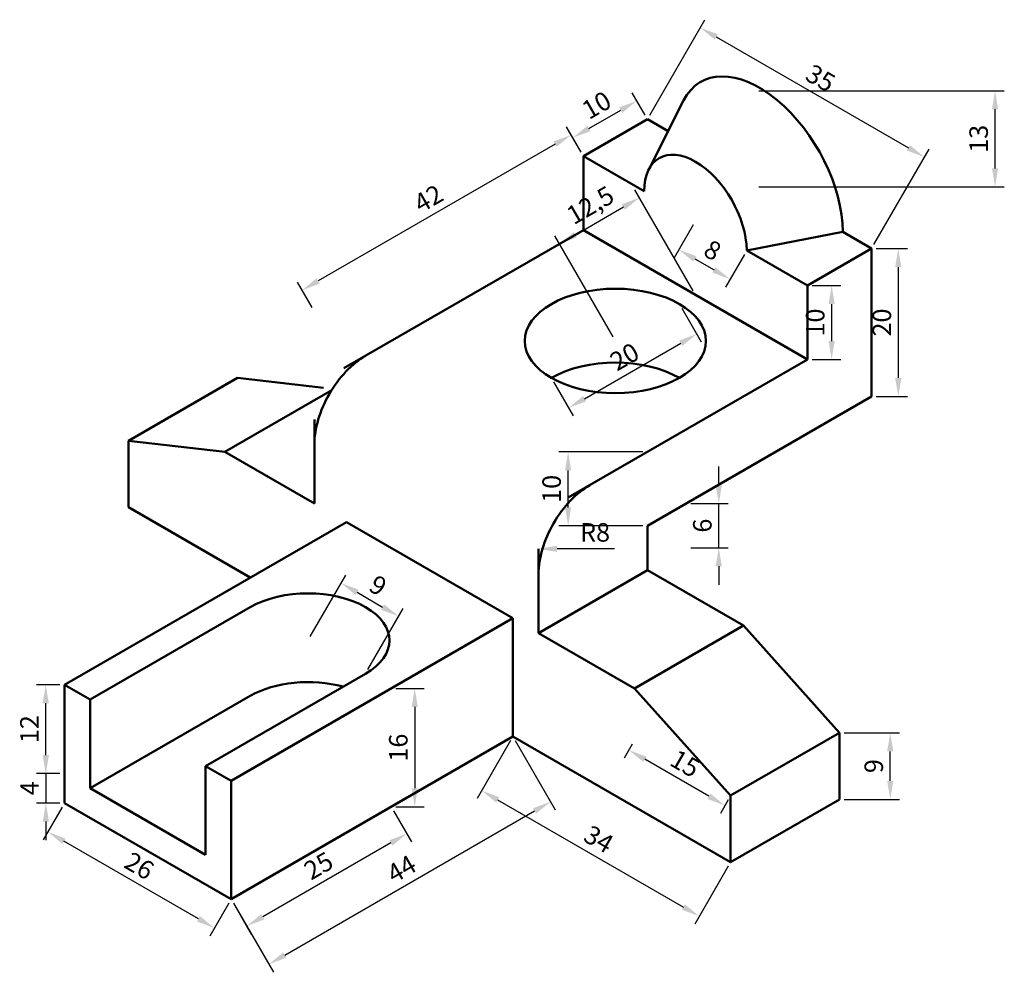
# Model space of a CAD drawing. Units: millimetres. Extents: x 1715 to 1848, y 1134 to 1263.
import ezdxf

# ---------------------------------------------------------------- set-up
doc = ezdxf.new("R2010")
doc.units = ezdxf.units.MM
doc.layers.add('M-DIMS', color=2, linetype='Continuous', lineweight=25)
doc.layers.add('M-OUTL', color=7, linetype='Continuous', lineweight=50)
doc.styles.get("Standard").update_dxf_attribs({"font": 'arial.ttf'})
doc.dimstyles.new('ISO-25', dxfattribs={"dimtxt": 2.5, "dimasz": 2.5, "dimexe": 1.25, "dimexo": 0.625, "dimtad": 1, "dimtxsty": 'Standard', "dimcen": 2.5, "dimadec": 0, "dimazin": 0, "dimtfac": 1, "dimtmove": 0, "dimatfit": 3, "dimfxl": 1, "dimarcsym": 0})

# ---------------------------------------------------------------- blocks, each defined once
blk = doc.blocks.new('*D1')
at = {"layer": 'Defpoints', "color": 0, "transparency": 16777216}
for p in [(1781.77, 1166.31), (1811.22, 1149.31), (1806.99, 1142)]:
    blk.add_point(p, dxfattribs=at)
at = {"layer": 'M-DIMS', "color": 0, "lineweight": -2, "transparency": 16777216}
for p, q in [((1781.46, 1165.77), (1776.92, 1157.92)), ((1779.71, 1157.75), (1804.83, 1143.25)), ((1810.9, 1148.77), (1806.37, 1140.92))]:
    blk.add_line(p, q, dxfattribs=at)
at = {"layer": 'M-DIMS', "color": 0, "transparency": 16777216}
for points in [[(1779.92, 1158.11), (1779.5, 1157.39), (1777.55, 1159)], [(1805.04, 1143.61), (1804.62, 1142.89), (1806.99, 1142)]]:
    blk.add_solid(points, dxfattribs=at)
at = {"layer": 'M-DIMS', "color": 0, "transparency": 16777216, "insert": (1793.22, 1152.15), "char_height": 2.5, "attachment_point": 5, "rotation": 330}
blk.add_mtext('34', dxfattribs=at)
blk = doc.blocks.new('*D2')
at = {"layer": 'Defpoints', "color": 0, "transparency": 16777216}
for p in [(1798.23, 1165.81), (1797.46, 1164.48), (1811.22, 1158.31)]:
    blk.add_point(p, dxfattribs=at)
at = {"layer": 'M-DIMS', "color": 0, "lineweight": -2, "transparency": 16777216}
for p, q in [((1797.91, 1165.27), (1796.83, 1163.4)), ((1808.28, 1158.23), (1799.62, 1163.23)), ((1810.9, 1157.77), (1809.82, 1155.9))]:
    blk.add_line(p, q, dxfattribs=at)
at = {"layer": 'M-DIMS', "color": 0, "transparency": 16777216}
for points in [[(1799.83, 1163.59), (1799.41, 1162.87), (1797.46, 1164.48)], [(1808.49, 1158.59), (1808.07, 1157.87), (1810.45, 1156.98)]]:
    blk.add_solid(points, dxfattribs=at)
at = {"layer": 'M-DIMS', "color": 0, "transparency": 16777216, "insert": (1804.9, 1162.38), "char_height": 2.5, "attachment_point": 5, "rotation": 330}
blk.add_mtext('15', dxfattribs=at)
blk = doc.blocks.new('*D3')
at = {"layer": 'Defpoints', "color": 0, "transparency": 16777216}
for p in [(1825.94, 1166.81), (1832.79, 1166.81), (1825.94, 1157.81)]:
    blk.add_point(p, dxfattribs=at)
at = {"layer": 'M-DIMS', "color": 0, "lineweight": -2, "transparency": 16777216}
for p, q in [((1826.56, 1166.81), (1834.04, 1166.81)), ((1832.79, 1160.31), (1832.79, 1164.31)), ((1826.56, 1157.81), (1834.04, 1157.81))]:
    blk.add_line(p, q, dxfattribs=at)
at = {"layer": 'M-DIMS', "color": 0, "transparency": 16777216}
for points in [[(1832.38, 1164.31), (1833.21, 1164.31), (1832.79, 1166.81)], [(1832.38, 1160.31), (1833.21, 1160.31), (1832.79, 1157.81)]]:
    blk.add_solid(points, dxfattribs=at)
at = {"layer": 'M-DIMS', "color": 0, "transparency": 16777216, "insert": (1830.89, 1162.31), "char_height": 2.5, "attachment_point": 5, "rotation": 90}
blk.add_mtext('9', dxfattribs=at)
blk = doc.blocks.new('*D4')
at = {"layer": 'Defpoints', "color": 0, "transparency": 16777216}
for p in [(1789.24, 1204.81), (1799.96, 1204.81), (1799.96, 1194.81)]:
    blk.add_point(p, dxfattribs=at)
at = {"layer": 'M-DIMS', "color": 0, "lineweight": -2, "transparency": 16777216}
for p, q in [((1799.33, 1204.81), (1787.99, 1204.81)), ((1789.24, 1197.31), (1789.24, 1202.31)), ((1799.33, 1194.81), (1787.99, 1194.81))]:
    blk.add_line(p, q, dxfattribs=at)
at = {"layer": 'M-DIMS', "color": 0, "transparency": 16777216}
for points in [[(1788.82, 1202.31), (1789.65, 1202.31), (1789.24, 1204.81)], [(1788.82, 1197.31), (1789.65, 1197.31), (1789.24, 1194.81)]]:
    blk.add_solid(points, dxfattribs=at)
at = {"layer": 'M-DIMS', "color": 0, "transparency": 16777216, "insert": (1787.33, 1199.81), "char_height": 2.5, "attachment_point": 5, "rotation": 90}
blk.add_mtext('10', dxfattribs=at)
blk = doc.blocks.new('*D5')
at = {"layer": 'Defpoints', "color": 0, "transparency": 16777216}
for p in [(1821.61, 1227.31), (1821.61, 1217.31), (1824.87, 1217.31)]:
    blk.add_point(p, dxfattribs=at)
at = {"layer": 'M-DIMS', "color": 0, "lineweight": -2, "transparency": 16777216}
for p, q in [((1822.23, 1227.31), (1826.12, 1227.31)), ((1824.87, 1224.81), (1824.87, 1219.81)), ((1822.23, 1217.31), (1826.12, 1217.31))]:
    blk.add_line(p, q, dxfattribs=at)
at = {"layer": 'M-DIMS', "color": 0, "transparency": 16777216}
for points in [[(1824.45, 1224.81), (1825.29, 1224.81), (1824.87, 1227.31)], [(1824.45, 1219.81), (1825.29, 1219.81), (1824.87, 1217.31)]]:
    blk.add_solid(points, dxfattribs=at)
at = {"layer": 'M-DIMS', "color": 0, "transparency": 16777216, "insert": (1822.97, 1222.31), "char_height": 2.5, "attachment_point": 5, "rotation": 90}
blk.add_mtext('10', dxfattribs=at)
blk = doc.blocks.new('*D6')
at = {"layer": 'Defpoints', "color": 0, "transparency": 16777216}
for p in [(1830.27, 1232.31), (1830.27, 1212.31), (1833.88, 1212.31)]:
    blk.add_point(p, dxfattribs=at)
at = {"layer": 'M-DIMS', "color": 0, "lineweight": -2, "transparency": 16777216}
for p, q in [((1830.89, 1232.31), (1835.13, 1232.31)), ((1833.88, 1229.81), (1833.88, 1214.81)), ((1830.89, 1212.31), (1835.13, 1212.31))]:
    blk.add_line(p, q, dxfattribs=at)
at = {"layer": 'M-DIMS', "color": 0, "transparency": 16777216}
for points in [[(1833.46, 1229.81), (1834.3, 1229.81), (1833.88, 1232.31)], [(1833.46, 1214.81), (1834.3, 1214.81), (1833.88, 1212.31)]]:
    blk.add_solid(points, dxfattribs=at)
at = {"layer": 'M-DIMS', "color": 0, "transparency": 16777216, "insert": (1831.98, 1222.31), "char_height": 2.5, "attachment_point": 5, "rotation": 90}
blk.add_mtext('20', dxfattribs=at)
blk = doc.blocks.new('*D7')
at = {"layer": 'Defpoints', "color": 0, "transparency": 16777216}
for p in [(1799.96, 1249.81), (1837.41, 1244.69), (1830.27, 1232.31)]:
    blk.add_point(p, dxfattribs=at)
at = {"layer": 'M-DIMS', "color": 0, "lineweight": -2, "transparency": 16777216}
for p, q in [((1800.27, 1250.36), (1807.73, 1263.27)), ((1809.27, 1260.94), (1835.25, 1245.94)), ((1830.58, 1232.86), (1838.04, 1245.77))]:
    blk.add_line(p, q, dxfattribs=at)
at = {"layer": 'M-DIMS', "color": 0, "transparency": 16777216}
for points in [[(1809.48, 1261.3), (1809.06, 1260.58), (1807.1, 1262.19)], [(1835.46, 1246.3), (1835.04, 1245.58), (1837.41, 1244.69)]]:
    blk.add_solid(points, dxfattribs=at)
at = {"layer": 'M-DIMS', "color": 0, "transparency": 16777216, "insert": (1823.21, 1255.09), "char_height": 2.5, "attachment_point": 5, "rotation": 330}
blk.add_mtext('35', dxfattribs=at)
blk = doc.blocks.new('*D8')
at = {"layer": 'Defpoints', "color": 0, "transparency": 16777216}
for p in [(1798.53, 1252.3), (1799.96, 1249.81), (1791.3, 1244.81)]:
    blk.add_point(p, dxfattribs=at)
at = {"layer": 'M-DIMS', "color": 0, "lineweight": -2, "transparency": 16777216}
for p, q in [((1799.65, 1250.36), (1797.9, 1253.38)), ((1792.03, 1248.55), (1796.36, 1251.05)), ((1790.99, 1245.36), (1789.24, 1248.38))]:
    blk.add_line(p, q, dxfattribs=at)
at = {"layer": 'M-DIMS', "color": 0, "transparency": 16777216}
for points in [[(1796.15, 1251.41), (1796.57, 1250.68), (1798.53, 1252.3)], [(1791.82, 1248.91), (1792.24, 1248.18), (1789.87, 1247.3)]]:
    blk.add_solid(points, dxfattribs=at)
at = {"layer": 'M-DIMS', "color": 0, "transparency": 16777216, "insert": (1793.24, 1251.44), "char_height": 2.5, "attachment_point": 5, "rotation": 30}
blk.add_mtext('10', dxfattribs=at)
blk = doc.blocks.new('*D9')
at = {"layer": 'Defpoints', "color": 0, "transparency": 16777216}
for p in [(1798.88, 1239.19), (1806.45, 1226.06), (1795.63, 1219.81)]:
    blk.add_point(p, dxfattribs=at)
at = {"layer": 'M-DIMS', "color": 0, "lineweight": -2, "transparency": 16777216}
for p, q in [((1806.14, 1226.61), (1798.25, 1240.27)), ((1790.22, 1234.19), (1796.71, 1237.94)), ((1795.32, 1220.36), (1787.43, 1234.02))]:
    blk.add_line(p, q, dxfattribs=at)
at = {"layer": 'M-DIMS', "color": 0, "transparency": 16777216}
for points in [[(1796.5, 1238.3), (1796.92, 1237.58), (1798.88, 1239.19)], [(1790.01, 1234.55), (1790.42, 1233.83), (1788.05, 1232.94)]]:
    blk.add_solid(points, dxfattribs=at)
at = {"layer": 'M-DIMS', "color": 0, "transparency": 16777216, "insert": (1792.4, 1237.91), "char_height": 2.5, "attachment_point": 5, "rotation": 30}
blk.add_mtext('12,5', dxfattribs=at)
blk = doc.blocks.new('*D10')
at = {"layer": 'Defpoints', "color": 0, "transparency": 16777216}
for p in [(1804.29, 1224.81), (1806.63, 1220.76), (1786.97, 1214.81)]:
    blk.add_point(p, dxfattribs=at)
at = {"layer": 'M-DIMS', "color": 0, "lineweight": -2, "transparency": 16777216}
for p, q in [((1804.6, 1224.27), (1807.25, 1219.68)), ((1791.47, 1212.01), (1804.46, 1219.51)), ((1787.28, 1214.27), (1789.93, 1209.68))]:
    blk.add_line(p, q, dxfattribs=at)
at = {"layer": 'M-DIMS', "color": 0, "transparency": 16777216}
for points in [[(1804.26, 1219.87), (1804.67, 1219.15), (1806.63, 1220.76)], [(1791.27, 1212.37), (1791.68, 1211.65), (1789.31, 1210.76)]]:
    blk.add_solid(points, dxfattribs=at)
at = {"layer": 'M-DIMS', "color": 0, "transparency": 16777216, "insert": (1797.02, 1217.41), "char_height": 2.5, "attachment_point": 5, "rotation": 30}
blk.add_mtext('20', dxfattribs=at)
blk = doc.blocks.new('*D11')
at = {"layer": 'Defpoints', "color": 0, "transparency": 16777216}
for p in [(1791.3, 1244.81), (1753.27, 1226.68), (1754.92, 1223.81)]:
    blk.add_point(p, dxfattribs=at)
at = {"layer": 'M-DIMS', "color": 0, "lineweight": -2, "transparency": 16777216}
for p, q in [((1790.99, 1245.36), (1789.02, 1248.77)), ((1787.48, 1246.43), (1755.43, 1227.93)), ((1754.61, 1224.36), (1752.64, 1227.77))]:
    blk.add_line(p, q, dxfattribs=at)
at = {"layer": 'M-DIMS', "color": 0, "transparency": 16777216}
for points in [[(1787.27, 1246.8), (1787.68, 1246.07), (1789.64, 1247.68)], [(1755.22, 1228.3), (1755.64, 1227.57), (1753.27, 1226.68)]]:
    blk.add_solid(points, dxfattribs=at)
at = {"layer": 'M-DIMS', "color": 0, "transparency": 16777216, "insert": (1770.51, 1238.81), "char_height": 2.5, "attachment_point": 5, "rotation": 30}
blk.add_mtext('42', dxfattribs=at)
blk = doc.blocks.new('*D12')
at = {"layer": 'Defpoints', "color": 0, "transparency": 16777216}
for p in [(1766.33, 1182.57), (1754.06, 1179.31), (1761.85, 1174.81)]:
    blk.add_point(p, dxfattribs=at)
at = {"layer": 'M-DIMS', "color": 0, "lineweight": -2, "transparency": 16777216}
for p, q in [((1754.37, 1179.86), (1759.16, 1188.15)), ((1760.7, 1185.82), (1764.16, 1183.82)), ((1762.17, 1175.36), (1766.95, 1183.65))]:
    blk.add_line(p, q, dxfattribs=at)
at = {"layer": 'M-DIMS', "color": 0, "transparency": 16777216}
for points in [[(1760.91, 1186.18), (1760.49, 1185.46), (1758.53, 1187.07)], [(1764.37, 1184.18), (1763.96, 1183.46), (1766.33, 1182.57)]]:
    blk.add_solid(points, dxfattribs=at)
at = {"layer": 'M-DIMS', "color": 0, "transparency": 16777216, "insert": (1763.38, 1186.46), "char_height": 2.5, "attachment_point": 5, "rotation": 330}
blk.add_mtext('9', dxfattribs=at)
blk = doc.blocks.new('*D13')
at = {"layer": 'Defpoints', "color": 0, "transparency": 16777216}
for p in [(1765.32, 1156.81), (1743.67, 1144.31), (1745.77, 1140.67)]:
    blk.add_point(p, dxfattribs=at)
at = {"layer": 'M-DIMS', "color": 0, "lineweight": -2, "transparency": 16777216}
for p, q in [((1765.63, 1156.27), (1768.05, 1152.08)), ((1765.26, 1151.92), (1747.94, 1141.92)), ((1743.98, 1143.77), (1746.4, 1139.58))]:
    blk.add_line(p, q, dxfattribs=at)
at = {"layer": 'M-DIMS', "color": 0, "transparency": 16777216}
for points in [[(1765.05, 1152.28), (1765.47, 1151.56), (1767.42, 1153.17)], [(1747.73, 1142.28), (1748.15, 1141.56), (1745.77, 1140.67)]]:
    blk.add_solid(points, dxfattribs=at)
at = {"layer": 'M-DIMS', "color": 0, "transparency": 16777216, "insert": (1755.65, 1148.56), "char_height": 2.5, "attachment_point": 5, "rotation": 30}
blk.add_mtext('25', dxfattribs=at)
blk = doc.blocks.new('*D14')
at = {"layer": 'Defpoints', "color": 0, "transparency": 16777216}
for p in [(1721.15, 1157.31), (1718.89, 1153.41), (1743.67, 1144.31)]:
    blk.add_point(p, dxfattribs=at)
at = {"layer": 'M-DIMS', "color": 0, "lineweight": -2, "transparency": 16777216}
for p, q in [((1720.84, 1156.77), (1718.27, 1152.32)), ((1739.24, 1141.66), (1721.06, 1152.16)), ((1743.35, 1143.77), (1740.78, 1139.32))]:
    blk.add_line(p, q, dxfattribs=at)
at = {"layer": 'M-DIMS', "color": 0, "transparency": 16777216}
for points in [[(1721.27, 1152.52), (1720.85, 1151.8), (1718.89, 1153.41)], [(1739.45, 1142.02), (1739.04, 1141.3), (1741.41, 1140.41)]]:
    blk.add_solid(points, dxfattribs=at)
at = {"layer": 'M-DIMS', "color": 0, "transparency": 16777216, "insert": (1731.1, 1148.55), "char_height": 2.5, "attachment_point": 5, "rotation": 330}
blk.add_mtext('26', dxfattribs=at)
blk = doc.blocks.new('*D15')
at = {"layer": 'Defpoints', "color": 0, "transparency": 16777216}
for p in [(1781.77, 1166.31), (1786.86, 1157.5), (1743.67, 1144.31)]:
    blk.add_point(p, dxfattribs=at)
at = {"layer": 'M-DIMS', "color": 0, "lineweight": -2, "transparency": 16777216}
for p, q in [((1782.08, 1165.77), (1787.48, 1156.42)), ((1750.92, 1136.75), (1784.69, 1156.25)), ((1743.98, 1143.77), (1749.38, 1134.42))]:
    blk.add_line(p, q, dxfattribs=at)
at = {"layer": 'M-DIMS', "color": 0, "transparency": 16777216}
for points in [[(1784.49, 1156.61), (1784.9, 1155.89), (1786.86, 1157.5)], [(1750.71, 1137.11), (1751.13, 1136.39), (1748.75, 1135.5)]]:
    blk.add_solid(points, dxfattribs=at)
at = {"layer": 'M-DIMS', "color": 0, "transparency": 16777216, "insert": (1766.87, 1148.13), "char_height": 2.5, "attachment_point": 5, "rotation": 30}
blk.add_mtext('44', dxfattribs=at)
blk = doc.blocks.new('*D16')
at = {"layer": 'Defpoints', "color": 0, "transparency": 16777216}
for p in [(1721.15, 1161.31), (1718.62, 1157.31), (1721.15, 1157.31)]:
    blk.add_point(p, dxfattribs=at)
at = {"layer": 'M-DIMS', "color": 0, "lineweight": -2, "transparency": 16777216}
for p, q in [((1718.62, 1163.81), (1718.62, 1166.31)), ((1720.52, 1161.31), (1717.37, 1161.31)), ((1718.62, 1161.31), (1718.62, 1157.31)), ((1720.52, 1157.31), (1717.37, 1157.31)), ((1718.62, 1154.81), (1718.62, 1152.31))]:
    blk.add_line(p, q, dxfattribs=at)
at = {"layer": 'M-DIMS', "color": 0, "transparency": 16777216}
for points in [[(1718.2, 1163.81), (1719.04, 1163.81), (1718.62, 1161.31)], [(1718.2, 1154.81), (1719.04, 1154.81), (1718.62, 1157.31)]]:
    blk.add_solid(points, dxfattribs=at)
at = {"layer": 'M-DIMS', "color": 0, "transparency": 16777216, "insert": (1716.74, 1159.31), "char_height": 2.5, "attachment_point": 5, "rotation": 90}
blk.add_mtext('4', dxfattribs=at)
blk = doc.blocks.new('*D17')
at = {"layer": 'Defpoints', "color": 0, "transparency": 16777216}
for p in [(1718.6, 1173.31), (1721.15, 1173.31), (1721.15, 1161.31)]:
    blk.add_point(p, dxfattribs=at)
at = {"layer": 'M-DIMS', "color": 0, "lineweight": -2, "transparency": 16777216}
for p, q in [((1720.52, 1173.31), (1717.35, 1173.31)), ((1718.6, 1163.81), (1718.6, 1170.81)), ((1720.52, 1161.31), (1717.35, 1161.31))]:
    blk.add_line(p, q, dxfattribs=at)
at = {"layer": 'M-DIMS', "color": 0, "transparency": 16777216}
for points in [[(1718.18, 1170.81), (1719.02, 1170.81), (1718.6, 1173.31)], [(1718.18, 1163.81), (1719.02, 1163.81), (1718.6, 1161.31)]]:
    blk.add_solid(points, dxfattribs=at)
at = {"layer": 'M-DIMS', "color": 0, "transparency": 16777216, "insert": (1716.72, 1167.31), "char_height": 2.5, "attachment_point": 5, "rotation": 90}
blk.add_mtext('12', dxfattribs=at)
blk = doc.blocks.new('*D18')
at = {"layer": 'Defpoints', "color": 0, "transparency": 16777216}
for p in [(1765.32, 1172.81), (1765.32, 1156.81), (1768.5, 1156.81)]:
    blk.add_point(p, dxfattribs=at)
at = {"layer": 'M-DIMS', "color": 0, "lineweight": -2, "transparency": 16777216}
for p, q in [((1765.94, 1172.81), (1769.75, 1172.81)), ((1768.5, 1170.31), (1768.5, 1159.31)), ((1765.94, 1156.81), (1769.75, 1156.81))]:
    blk.add_line(p, q, dxfattribs=at)
at = {"layer": 'M-DIMS', "color": 0, "transparency": 16777216}
for points in [[(1768.08, 1170.31), (1768.92, 1170.31), (1768.5, 1172.81)], [(1768.08, 1159.31), (1768.92, 1159.31), (1768.5, 1156.81)]]:
    blk.add_solid(points, dxfattribs=at)
at = {"layer": 'M-DIMS', "color": 0, "transparency": 16777216, "insert": (1766.6, 1164.81), "char_height": 2.5, "attachment_point": 5, "rotation": 90}
blk.add_mtext('16', dxfattribs=at)
blk = doc.blocks.new('*D19')
at = {"layer": 'Defpoints', "color": 0, "transparency": 16777216}
for p in [(1785.24, 1191.7), (1793.24, 1191.7)]:
    blk.add_point(p, dxfattribs=at)
at = {"layer": 'M-DIMS', "color": 0, "lineweight": -2, "transparency": 16777216}
blk.add_line((1795.52, 1191.7), (1787.74, 1191.7), dxfattribs=at)
at = {"layer": 'M-DIMS', "color": 0, "transparency": 16777216}
blk.add_solid([(1787.74, 1192.11), (1787.74, 1191.28), (1785.24, 1191.7)], dxfattribs=at)
at = {"layer": 'M-DIMS', "color": 0, "transparency": 16777216, "insert": (1792.88, 1193.6), "char_height": 2.5, "attachment_point": 5}
blk.add_mtext('R8', dxfattribs=at)
blk = doc.blocks.new('*D20')
at = {"layer": 'Defpoints', "color": 0, "transparency": 16777216}
for p in [(1806.45, 1236.06), (1813.38, 1232.06), (1811.13, 1228.17)]:
    blk.add_point(p, dxfattribs=at)
at = {"layer": 'M-DIMS', "color": 0, "lineweight": -2, "transparency": 16777216}
for p, q in [((1806.14, 1235.52), (1803.58, 1231.08)), ((1813.07, 1231.52), (1810.51, 1227.08)), ((1806.37, 1230.92), (1808.97, 1229.42))]:
    blk.add_line(p, q, dxfattribs=at)
at = {"layer": 'M-DIMS', "color": 0, "transparency": 16777216}
for points in [[(1806.58, 1231.28), (1806.16, 1230.56), (1804.2, 1232.17)], [(1809.17, 1229.78), (1808.76, 1229.06), (1811.13, 1228.17)]]:
    blk.add_solid(points, dxfattribs=at)
at = {"layer": 'M-DIMS', "color": 0, "transparency": 16777216, "insert": (1808.62, 1231.81), "char_height": 2.5, "attachment_point": 5, "rotation": 330}
blk.add_mtext('8', dxfattribs=at)
blk = doc.blocks.new('*D21')
at = {"layer": 'Defpoints', "color": 0, "transparency": 16777216}
for p in [(1814.41, 1253.66), (1846.97, 1253.66), (1814.41, 1240.66)]:
    blk.add_point(p, dxfattribs=at)
at = {"layer": 'M-DIMS', "color": 0, "lineweight": -2, "transparency": 16777216}
for p, q in [((1815.04, 1253.66), (1848.22, 1253.66)), ((1846.97, 1243.16), (1846.97, 1251.16)), ((1815.04, 1240.66), (1848.22, 1240.66))]:
    blk.add_line(p, q, dxfattribs=at)
at = {"layer": 'M-DIMS', "color": 0, "transparency": 16777216}
for points in [[(1846.55, 1251.16), (1847.38, 1251.16), (1846.97, 1253.66)], [(1846.55, 1243.16), (1847.38, 1243.16), (1846.97, 1240.66)]]:
    blk.add_solid(points, dxfattribs=at)
at = {"layer": 'M-DIMS', "color": 0, "transparency": 16777216, "insert": (1845.07, 1247.16), "char_height": 2.5, "attachment_point": 5, "rotation": 90}
blk.add_mtext('13', dxfattribs=at)
blk = doc.blocks.new('*D22')
at = {"layer": 'Defpoints', "color": 0, "transparency": 16777216}
for p in [(1805.2, 1197.84), (1809.61, 1197.84), (1805.2, 1191.84)]:
    blk.add_point(p, dxfattribs=at)
at = {"layer": 'M-DIMS', "color": 0, "lineweight": -2, "transparency": 16777216}
for p, q in [((1809.61, 1200.34), (1809.61, 1202.84)), ((1805.82, 1197.84), (1810.86, 1197.84)), ((1809.61, 1191.84), (1809.61, 1197.84)), ((1805.82, 1191.84), (1810.86, 1191.84)), ((1809.61, 1189.34), (1809.61, 1186.84))]:
    blk.add_line(p, q, dxfattribs=at)
at = {"layer": 'M-DIMS', "color": 0, "transparency": 16777216}
for points in [[(1809.19, 1200.34), (1810.03, 1200.34), (1809.61, 1197.84)], [(1809.19, 1189.34), (1810.03, 1189.34), (1809.61, 1191.84)]]:
    blk.add_solid(points, dxfattribs=at)
at = {"layer": 'M-DIMS', "color": 0, "transparency": 16777216, "insert": (1807.71, 1194.84), "char_height": 2.5, "attachment_point": 5, "rotation": 90}
blk.add_mtext('6', dxfattribs=at)

msp = doc.modelspace()

# ---------------------------------------------------------------- linework, layer by layer
at = {"layer": 'M-OUTL'}
for p, q in [((1800.139, 1243.002), (1804.852, 1252.338)), ((1799.958, 1249.815), (1791.298, 1244.815)), ((1802.761, 1248.196), (1799.958, 1249.815)), ((1791.298, 1234.815), (1791.298, 1244.815)), ((1799.525, 1240.065), (1791.298, 1244.815)), ((1791.298, 1234.815), (1758.925, 1216.124)), ((1821.609, 1217.315), (1791.298, 1234.815)), ((1813.381, 1232.065), (1826.372, 1234.565)), ((1830.269, 1232.315), (1826.372, 1234.565)), ((1821.609, 1227.315), (1813.381, 1232.065)), ((1821.609, 1227.315), (1830.269, 1232.315)), ((1830.269, 1232.315), (1830.269, 1212.315)), ((1821.609, 1217.315), (1821.609, 1227.315)), ((1789.236, 1198.624), (1821.609, 1217.315)), ((1744.532, 1214.815), (1729.81, 1206.315)), ((1756.163, 1213.472), (1744.532, 1214.815)), ((1742.8, 1204.815), (1757.27, 1213.169)), ((1742.8, 1204.815), (1755.486, 1212.138)), ((1830.269, 1212.315), (1799.958, 1194.815)), ((1754.925, 1209.196), (1754.925, 1197.815)), ((1729.81, 1197.315), (1729.81, 1206.315)), ((1729.81, 1206.315), (1742.8, 1204.815)), ((1754.925, 1197.815), (1742.8, 1204.815)), ((1746.264, 1187.815), (1729.81, 1197.315)), ((1721.15, 1173.315), (1759.255, 1195.315)), ((1781.771, 1182.315), (1759.255, 1195.315)), ((1799.958, 1194.815), (1799.958, 1188.815)), ((1785.236, 1180.315), (1785.236, 1191.696)), ((1785.236, 1180.315), (1799.958, 1188.815)), ((1812.948, 1181.315), (1799.958, 1188.815)), ((1743.666, 1160.315), (1781.771, 1182.315)), ((1781.771, 1182.315), (1781.771, 1166.315)), ((1781.771, 1182.315), (1781.771, 1182.315)), ((1798.226, 1172.815), (1812.948, 1181.315)), ((1825.939, 1166.815), (1812.948, 1181.315)), ((1785.236, 1180.315), (1798.226, 1172.815)), ((1740.202, 1162.315), (1761.853, 1174.815)), ((1721.15, 1161.315), (1721.15, 1173.315)), ((1721.15, 1173.315), (1724.614, 1171.315)), ((1724.614, 1159.315), (1746.264, 1171.815)), ((1798.226, 1172.815), (1811.216, 1158.315)), ((1724.614, 1171.315), (1724.614, 1159.315)), ((1743.666, 1144.315), (1781.771, 1166.315)), ((1781.771, 1166.315), (1811.216, 1149.315)), ((1811.216, 1158.315), (1825.939, 1166.815)), ((1825.939, 1166.815), (1825.939, 1157.815)), ((1740.202, 1150.315), (1740.202, 1162.315)), ((1740.202, 1162.315), (1743.666, 1160.315)), ((1721.15, 1157.315), (1721.15, 1161.315)), ((1743.666, 1160.315), (1743.666, 1144.315)), ((1724.614, 1159.315), (1740.202, 1150.315)), ((1811.216, 1149.315), (1811.216, 1158.315)), ((1743.666, 1144.315), (1721.15, 1157.315)), ((1825.939, 1157.815), (1811.216, 1149.315))]:
    msp.add_line(p, q, dxfattribs=at)
msp.add_lwpolyline([(1724.614, 1171.315), (1746.264, 1183.815)], dxfattribs=at)
for centre, major_axis, start_param, end_param in [((1815.113, 1241.065), (7.961, -13.789), 0.7853982, 3.5029598), ((1806.453, 1236.065), (4.899, -8.485), 0.7853982, 3.9269908), ((1761.852, 1209.815), (-4.899, -8.485), 3.9269286, 5.4978493), ((1795.628, 1209.815), (12.247, 0), 0.7853982, 2.3561945), ((1792.163, 1192.315), (-4.899, -8.485), 3.9269286, 5.4978493), ((1754.059, 1179.315), (-11.023, 0), 2.3561945, 5.4977871), ((1754.059, 1167.315), (-11.023, 0), 4.2668277, 5.4977871)]:
    msp.add_ellipse(centre, major_axis=major_axis, ratio=0.5773503, start_param=start_param, end_param=end_param, dxfattribs=at)
msp.add_ellipse((1795.628, 1219.815), major_axis=(-12.247, 0), ratio=0.5773503, dxfattribs=at)

# ---------------------------------------------------------------- dimensions: what is measured, and where the dimension line sits
at = {"layer": 'M-DIMS'}
for p1, p2, distance, picture, middle in [((1799.958, 1249.815), (1830.269, 1232.315), 14.289, '*D7', (1823.209, 1255.086)), ((1791.298, 1244.815), (1799.958, 1249.815), 2.864, '*D8', (1793.245, 1251.442)), ((1791.298, 1244.815), (1754.925, 1223.815), -3.314, '*D11', (1770.514, 1238.813)), ((1795.628, 1219.815), (1806.453, 1226.065), 15.155, '*D9', (1792.399, 1237.907)), ((1806.453, 1236.065), (1813.381, 1232.065), -4.5, '*D20', (1808.618, 1231.814)), ((1786.968, 1214.815), (1804.288, 1224.815), -4.683, '*D10', (1797.018, 1217.406)), ((1754.059, 1179.315), (1761.853, 1174.815), 8.952, '*D12', (1763.383, 1186.464)), ((1743.666, 1144.315), (1781.771, 1166.315), -10.174, '*D15', (1766.869, 1148.127)), ((1781.771, 1166.315), (1811.216, 1149.315), -8.447, '*D1', (1793.222, 1152.147)), ((1811.216, 1158.315), (1798.226, 1165.815), 1.54, '*D2', (1804.902, 1162.377)), ((1743.666, 1144.315), (1721.15, 1157.315), 4.513, '*D14', (1731.102, 1148.553)), ((1765.317, 1156.815), (1743.666, 1144.315), 4.213, '*D13', (1755.647, 1148.563))]:
    dim = msp.add_aligned_dim(p1=p1, p2=p2, distance=distance, dimstyle='ISO-25', override={"dimclrd": 0, "dimclre": 0, "dimclrt": 0}, dxfattribs=at)
    dim.commit()
    dim.dimension.update_dxf_attribs({"geometry": picture, "text_midpoint": middle})
for base, p1, p2, picture, middle in [((1846.968, 1253.661), (1814.414, 1240.661), (1814.414, 1253.661), '*D21', (1845.065, 1247.161)), ((1833.882, 1212.315), (1830.269, 1232.315), (1830.269, 1212.315), '*D6', (1831.98, 1222.315)), ((1824.87, 1217.315), (1821.609, 1227.315), (1821.609, 1217.315), '*D5', (1822.969, 1222.315)), ((1789.236, 1204.815), (1799.958, 1194.815), (1799.958, 1204.815), '*D4', (1787.334, 1199.815)), ((1809.609, 1197.84), (1805.198, 1191.84), (1805.198, 1197.84), '*D22', (1807.707, 1194.84)), ((1718.601, 1173.315), (1721.15, 1161.315), (1721.15, 1173.315), '*D17', (1716.721, 1167.315)), ((1768.501, 1156.815), (1765.317, 1172.815), (1765.317, 1156.815), '*D18', (1766.6, 1164.815)), ((1718.618, 1157.315), (1721.15, 1161.315), (1721.15, 1157.315), '*D16', (1716.743, 1159.315)), ((1832.793, 1166.815), (1825.939, 1157.815), (1825.939, 1166.815), '*D3', (1830.891, 1162.315))]:
    dim = msp.add_linear_dim(base=base, p1=p1, p2=p2, angle=90, dimstyle='ISO-25', override={"dimclrd": 0, "dimclre": 0, "dimclrt": 0}, dxfattribs=at)
    dim.commit()
    dim.dimension.update_dxf_attribs({"geometry": picture, "text_midpoint": middle})
dim = msp.add_radius_dim(center=(1793.236, 1191.696), mpoint=(1785.236, 1191.696), dimstyle='ISO-25', override={"dimclrd": 0, "dimclre": 0, "dimclrt": 0}, dxfattribs=at)
dim.commit()
dim.dimension.update_dxf_attribs({"geometry": '*D19', "text_midpoint": (1792.879, 1191.696), "dimtype": 164})

doc.saveas('drawing.dxf')
